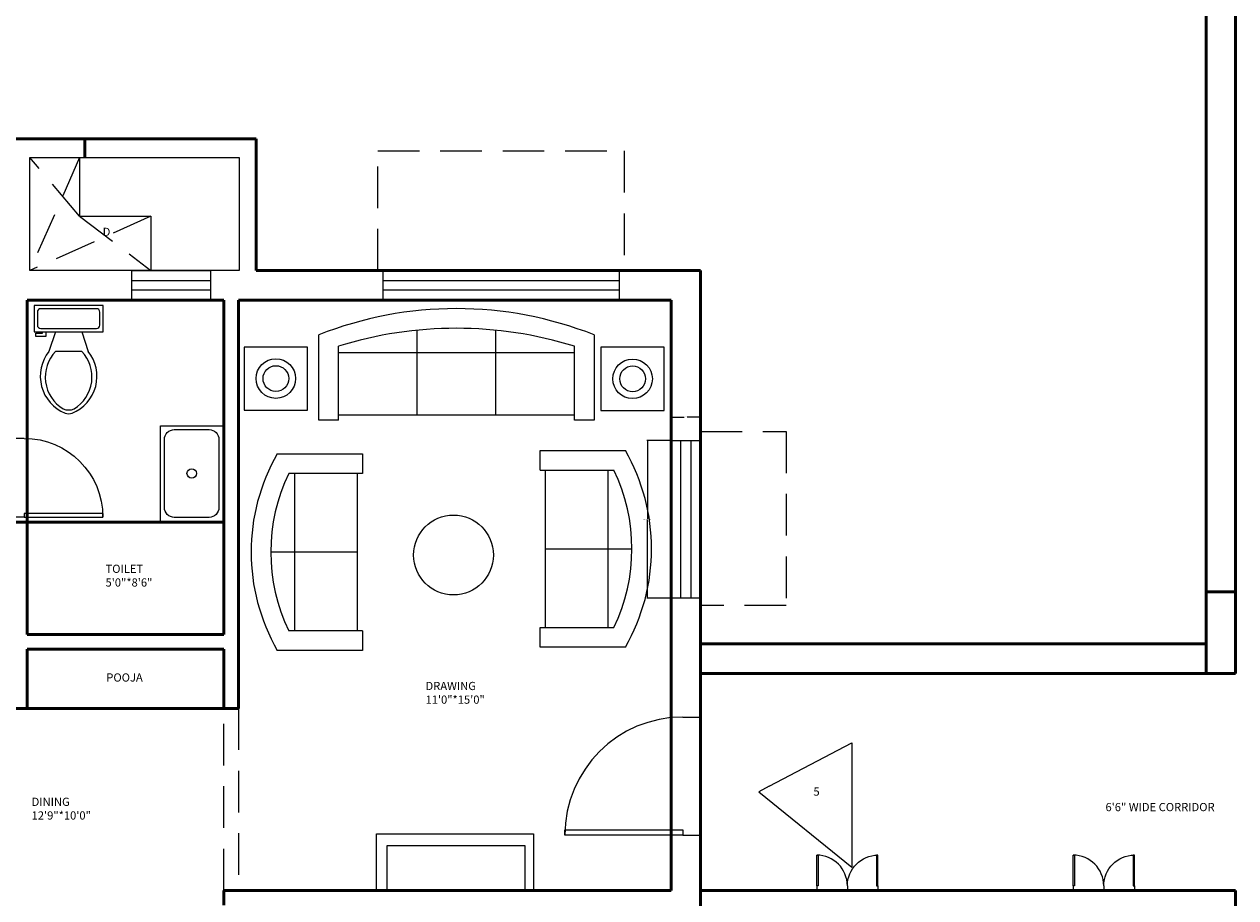
# Model space of a CAD drawing. Units: inches. Extents: x 4795 to 6024, y 2716 to 5025.
# Tile 6 of 19: x 5081 to 5450, y 3549 to 3816. Entities that reach past the tile are written whole.
import ezdxf

# ---------------------------------------------------------------- set-up
doc = ezdxf.new("R2010")
doc.units = ezdxf.units.IN
doc.linetypes.add('DASHED', pattern=[19.05, 12.7, -6.35])
for name, color, linetype, lineweight in [('A-ANNO-DIMS', 2, 'Continuous', 18), ('A-ANNO-TEXT', 7, 'Continuous', 18), ('A-AREA-IDEN', 3, 'Continuous', 18), ('A-DOOR', 4, 'Continuous', 25), ('A-FLOR-FIXT', 9, 'Continuous', 18), ('A-FURN', 8, 'Continuous', 18), ('A-GLAZ', 4, 'Continuous', 25), ('A-WALL', 7, 'Continuous', 50), ('A-WALL-OVHD', 8, 'DASHED', 18)]:
    doc.layers.add(name, color=color, linetype=linetype, lineweight=lineweight)
doc.styles.get("Standard").update_dxf_attribs({"font": 'arial.ttf'})
doc.dimstyles.get("Standard").update_dxf_attribs({"dimtxt": 0.18, "dimasz": 0.18, "dimexe": 0.18, "dimexo": 0.0625, "dimgap": 0.09, "dimtad": 0, "dimtih": 1, "dimtoh": 1, "dimdec": 4, "dimzin": 0, "dimdsep": 46, "dimtxsty": 'Standard', "dimcen": 0.09, "dimadec": 0, "dimazin": 0, "dimtfac": 1, "dimtdec": 4, "dimtofl": 0, "dimtmove": 0, "dimatfit": 3, "dimfxl": 1, "dimtolj": 1, "dimtzin": 0, "dimarcsym": 0})

# ---------------------------------------------------------------- blocks, each defined once
blk = doc.blocks.new('*U2')
for p, q in [((0, 0), (0, -6)), ((40, 0), (40, -6))]:
    blk.add_line(p, q)
blk.add_lwpolyline([(0, 0), (0, 40), (1.75, 40), (1.75, 0)], close=True)
blk.add_arc((0, 0), 40, 0, 90)
blk = doc.blocks.new('Sofa - Roundback 7 ft.')
for p, q in [((-12.00002, -32.4421), (-12.00003, -6.5971)), ((11.99997, -32.4421), (11.99998, -6.5971)), ((-36.000027, -34), (-36.000027, -11.4696)), ((-35.999844, -13.3819), (35.9998, -13.3819)), ((35.99998, -34), (35.99998, -11.4696)), ((-36.000027, -32.4421), (35.99998, -32.4421))]:
    blk.add_line(p, q)
for points in [[(-36.000027, -34), (-42.000027, -34), (-42.000027, -8)], [(41.99998, -8), (41.99998, -34), (35.99998, -34)]]:
    blk.add_lwpolyline(points)
for centre, radius, start, end in [((0, -114.25), 114.25, 68.43141, 111.5686), ((-0.00001, -127.1968), 121.1968, 72.72033, 107.2797)]:
    blk.add_arc(centre, radius, start, end)
blk = doc.blocks.new('Sofa - Roundback Loveseat 5 ft.')
for p, q in [((0, -32.44198), (0, -5.99998)), ((-24, -33.99998), (-24, -11.46958)), ((-23.9998, -13.38178), (23.99986, -13.38178)), ((24.00004, -33.99998), (24.00004, -11.46958)), ((-24, -32.44198), (24.00004, -32.44198))]:
    blk.add_line(p, q)
for points in [[(-24, -33.99998), (-30, -33.99998), (-30, -7.99998)], [(30.00004, -7.99998), (30.00004, -33.99998), (24.00004, -33.99998)]]:
    blk.add_lwpolyline(points)
for centre, radius, start, end in [((0, -60.24998), 60.24998, 60.13715, 119.8628), ((0, -61.38438), 55.38444, 64.32083, 115.6792)]:
    blk.add_arc(centre, radius, start, end)
blk = doc.blocks.new('Toilet - top')
for p, q in [((9.5, -6), (9.5, -2)), ((-10, -8.5), (-8, -8.5)), ((-10, -9.5), (-10, -8.5)), ((-7, -9.5), (-10, -9.5)), ((-8, -8.5), (-8, -8)), ((-7, -8), (-7, -9.5)), ((-4, -8), (-6, -14)), ((4, -8), (6, -14)), ((4, -14), (-4, -14))]:
    blk.add_line(p, q)
blk.add_lwpolyline([(10.5, -8), (10.5, 0), (-10.5, 0), (-10.5, -8)], close=True)
for points in [[(-9.5, -2), (-9.5, -6)], [(8.5, -1), (-8.5, -1)], [(-8.5, -7), (8.5, -7)]]:
    blk.add_lwpolyline(points)
for centre, radius, start, end in [((-8.62, -1.88), 0.884, 81.8699, 188.1301), ((8.62, -1.88), 0.884, 351.8699, 98.1301), ((-8.62, -6.12), 0.884, 171.8699, 278.1301), ((8.62, -6.12), 0.884, 261.8699, 8.1301), ((3.52, -21.58), 12.17, 141.4691, 247.9714), ((4.2, -21.82), 11.33, 136.3677, 238.9468), ((-3.52, -21.58), 12.17, 292.0284, 38.5307), ((-4.2, -21.82), 11.33, 301.053, 43.6321), ((0, -27.88), 4, 245.7318, 294.2682), ((0, -29), 4, 254.8605, 285.1395)]:
    blk.add_arc(centre, radius, start, end)
blk = doc.blocks.new('WIN-48')
for p, q in [((0, 0), (0, 48)), ((0, 48), (9, 48)), ((3, 0), (3, 48)), ((6, 48), (6, 0)), ((9, 48), (9, 0)), ((9, 0), (0, 0))]:
    blk.add_line(p, q)
blk = doc.blocks.new('WIN-72')
for p, q in [((0, 0), (0, 9)), ((0, 9), (72, 9)), ((72, 9), (72, 0)), ((0, 6), (72, 6)), ((72, 3), (0, 3)), ((72, 0), (0, 0))]:
    blk.add_line(p, q)
blk = doc.blocks.new('WIN-24')
for p, q in [((0, 0), (0, 9)), ((0, 9), (24, 9)), ((24, 9), (24, 0)), ((0, 6), (24, 6)), ((24, 3), (0, 3)), ((24, 0), (0, 0))]:
    blk.add_line(p, q)
blk = doc.blocks.new('*D35')
at = {"layer": 'A-ANNO-DIMS', "color": 0, "lineweight": -2, "transparency": 16777216}
for p, q in [((5277.91, 3688.56), (5270.59, 3688.56)), ((5270.77, 3688.38), (5270.77, 3664.74)), ((5270.77, 3640.74), (5270.77, 3664.38)), ((5277.91, 3640.56), (5270.59, 3640.56))]:
    blk.add_line(p, q, dxfattribs=at)
at = {"layer": 'A-ANNO-DIMS', "color": 0, "lineweight": 100, "transparency": 16777216}
for points in [[(5270.74, 3688.38), (5270.8, 3688.38), (5270.77, 3688.56)], [(5270.74, 3640.74), (5270.8, 3640.74), (5270.77, 3640.56)]]:
    blk.add_solid(points, dxfattribs=at)
at = {"layer": 'DEFPOINTS', "color": 0, "lineweight": 100, "transparency": 16777216}
for p in [(5277.97, 3688.56), (5270.77, 3640.56), (5277.97, 3640.56)]:
    blk.add_point(p, dxfattribs=at)
at = {"layer": 'A-ANNO-DIMS', "color": 0, "transparency": 16777216, "insert": (5270.77, 3664.56), "char_height": 0.18, "attachment_point": 5}
blk.add_mtext('\\A1;WINDOW 4\'-0" 48 TYP.', dxfattribs=at)
blk = doc.blocks.new('*D36')
at = {"layer": 'A-ANNO-DIMS', "color": 0, "lineweight": -2, "transparency": 16777216}
for p, q in [((5277.97, 3688.62), (5277.97, 3695.94)), ((5278.15, 3695.76), (5282.01, 3695.76)), ((5286.79, 3695.76), (5282.93, 3695.76)), ((5286.97, 3688.62), (5286.97, 3695.94))]:
    blk.add_line(p, q, dxfattribs=at)
at = {"layer": 'A-ANNO-DIMS', "color": 0, "lineweight": 100, "transparency": 16777216}
for points in [[(5278.15, 3695.79), (5278.15, 3695.73), (5277.97, 3695.76)], [(5286.79, 3695.79), (5286.79, 3695.73), (5286.97, 3695.76)]]:
    blk.add_solid(points, dxfattribs=at)
at = {"layer": 'DEFPOINTS', "color": 0, "lineweight": 100, "transparency": 16777216}
for p in [(5277.97, 3695.76), (5277.97, 3688.56), (5286.97, 3688.56)]:
    blk.add_point(p, dxfattribs=at)
at = {"layer": 'A-ANNO-DIMS', "color": 0, "transparency": 16777216, "insert": (5282.47, 3695.76), "char_height": 0.18, "attachment_point": 5}
blk.add_mtext('\\A1;9 TYP.', dxfattribs=at)

msp = doc.modelspace()

# ---------------------------------------------------------------- linework, layer by layer
at = {"layer": 'A-FLOR-FIXT'}
msp.add_lwpolyline([(5141.47, 3663.74), (5122.16, 3663.74), (5122.16, 3693.07), (5141.47, 3693.07)], close=True, dxfattribs=at)
msp.add_lwpolyline([(5126.37, 3691.93), (5136.99, 3691.93, -0.414214), (5139.99, 3688.93), (5139.99, 3668.17, -0.414214), (5136.99, 3665.17), (5126.37, 3665.17, -0.414214), (5123.37, 3668.17), (5123.37, 3688.93, -0.414214)], format="xyb", close=True, dxfattribs=at)
msp.add_circle((5131.68, 3678.55), 1.44, dxfattribs=at)
at = {"layer": 'A-FURN'}
for p, q in [((5082.32, 3740.43), (5082.32, 3774.86)), ((5082.32, 3774.86), (5146.16, 3774.86)), ((5097.44, 3774.86), (5097.44, 3757.06)), ((5146.16, 3774.86), (5146.16, 3740.43)), ((5097.44, 3757.06), (5119.25, 3757.06)), ((5119.25, 3757.06), (5119.25, 3740.43)), ((5146.16, 3740.43), (5082.32, 3740.43)), ((5307.95, 3583.17), (5333.15, 3596.44)), ((5333.15, 3596.44), (5333.15, 3558.52)), ((5307.95, 3583.17), (5304.79, 3581.51)), ((5304.79, 3581.51), (5333.15, 3558.52)), ((5188.04, 3551.43), (5188.04, 3568.62)), ((5188.04, 3568.62), (5236.04, 3568.62)), ((5236.04, 3568.62), (5236.04, 3551.43)), ((5191.33, 3551.43), (5191.33, 3565.1)), ((5191.33, 3565.1), (5233.37, 3565.1)), ((5233.37, 3565.1), (5233.37, 3551.43))]:
    msp.add_line(p, q, dxfattribs=at)
for points in [[(5167.05, 3717.11), (5147.69, 3717.11), (5147.69, 3697.86), (5167.05, 3697.86)], [(5275.91, 3717.03), (5256.55, 3717.03), (5256.55, 3697.78), (5275.91, 3697.78)]]:
    msp.add_lwpolyline(points, close=True, dxfattribs=at)
for centre, radius in [((5157.37, 3707.49), 6.04), ((5266.23, 3707.41), 6.04), ((5157.37, 3707.49), 3.92), ((5266.23, 3707.41), 3.92), ((5211.58, 3653.69), 12.16)]:
    msp.add_circle(centre, radius, dxfattribs=at)
at = {"layer": 'A-WALL'}
for p, q in [((5450.22, 4167.14), (5450.22, 3676.49)), ((5441.22, 4158.14), (5441.22, 3676.49)), ((5076.97, 3780.56), (5151.39, 3780.56)), ((5099.08, 3780.56), (5099.08, 3774.86)), ((5151.39, 3780.56), (5151.39, 3740.43)), ((5286.97, 3740.43), (5151.39, 3740.43)), ((5286.97, 3740.43), (5286.97, 3350.43)), ((5081.47, 3731.43), (5081.47, 3629.43)), ((5141.47, 3731.43), (5081.47, 3731.43)), ((5141.47, 3731.43), (5141.47, 3629.43)), ((5277.97, 3731.43), (5145.97, 3731.43)), ((5145.97, 3731.43), (5145.97, 3606.93)), ((5277.97, 3731.43), (5277.97, 3551.43)), ((5441.22, 3676.49), (5441.22, 3626.6)), ((5450.22, 3676.49), (5450.22, 3617.6)), ((5076.97, 3663.74), (5141.47, 3663.74)), ((5441.22, 3642.5), (5450.3, 3642.5)), ((5141.47, 3629.43), (5081.47, 3629.43)), ((5141.47, 3624.93), (5081.47, 3624.93)), ((5081.47, 3624.93), (5081.47, 3606.93)), ((5141.47, 3624.93), (5141.47, 3606.93)), ((5441.22, 3626.6), (5286.97, 3626.6)), ((5441.22, 3626.6), (5441.22, 3617.6)), ((5450.22, 3617.6), (5286.97, 3617.6)), ((5081.47, 3606.93), (5074.88, 3606.93)), ((5081.47, 3606.93), (5145.97, 3606.93)), ((5277.97, 3551.43), (5141.47, 3551.43)), ((5141.47, 3551.43), (5141.47, 3546.93)), ((5286.97, 3551.43), (5450.22, 3551.43)), ((5450.22, 3551.43), (5450.22, 3464.24))]:
    msp.add_line(p, q, dxfattribs=at)
at = {"layer": 'A-WALL-OVHD'}
for p, q in [((5097.44, 3757.06), (5082.32, 3774.86)), ((5097.44, 3774.86), (5082.32, 3740.43)), ((5188.49, 3740.43), (5188.49, 3776.92)), ((5188.49, 3776.92), (5263.68, 3776.92)), ((5263.68, 3776.92), (5263.68, 3740.43)), ((5119.25, 3757.06), (5082.32, 3740.43)), ((5097.44, 3757.06), (5119.25, 3740.43)), ((5286.97, 3691.35), (5313.11, 3691.35)), ((5313.11, 3691.35), (5313.11, 3638.32)), ((5313.11, 3638.32), (5286.97, 3638.32)), ((5141.47, 3551.43), (5141.47, 3606.93)), ((5145.97, 3606.93), (5145.97, 3551.43))]:
    msp.add_line(p, q, dxfattribs=at)

# ---------------------------------------------------------------- block references
at = {"layer": 'A-DOOR'}
for p, xscale, yscale, zscale, rotation in [((5080.57, 3665.26), -0.6, 0.6, 0.6, 270), ((5281.57, 3568.28), 0.9, 0.9, 0.9, 90)]:
    msp.add_blockref('*U2', p, dxfattribs=dict(at, xscale=xscale, yscale=yscale, zscale=zscale, rotation=rotation))
at = {"layer": 'A-DOOR', "yscale": 0.2337145210718518, "zscale": 0.2337145210718518}
for p, xscale in [((5322.42, 3552.81), 0.2337145210718518), ((5341.12, 3552.81), -0.2337145210718518), ((5400.66, 3552.81), 0.2337145210718518), ((5419.35, 3552.81), -0.2337145210718518)]:
    msp.add_blockref('*U2', p, dxfattribs=dict(at, xscale=xscale))
at = {"layer": 'A-FLOR-FIXT'}
msp.add_blockref('Toilet - top', (5094.13, 3729.79), dxfattribs=at)
at = {"layer": 'A-FURN'}
msp.add_blockref('Sofa - Roundback 7 ft.', (5212.46, 3728.83), dxfattribs=at)
for p, rotation in [((5149.81, 3654.59), 90), ((5272.02, 3655.57), 270)]:
    msp.add_blockref('Sofa - Roundback Loveseat 5 ft.', p, dxfattribs=dict(at, rotation=rotation))
at = {"layer": 'A-GLAZ', "rotation": 180}
for name, p in [('WIN-24', (5137.43, 3740.43)), ('WIN-72', (5262.11, 3740.43)), ('WIN-48', (5286.97, 3688.56))]:
    msp.add_blockref(name, p, dxfattribs=at)

# ---------------------------------------------------------------- texts
at = {"layer": 'A-ANNO-TEXT', "char_height": 2.5, "attachment_point": 1}
for s, width, insert in [('D', 2.4843, (5104.52, 3753.49)), ('5', 9.3052, (5321.42, 3582.79))]:
    msp.add_mtext_dynamic_manual_height_columns(s, width=width, gutter_width=12.5, heights=[0], dxfattribs=dict(at, insert=insert))
at = {"layer": 'A-AREA-IDEN', "char_height": 2.5, "attachment_point": 1}
for s, width, insert in [('TOILET\\P5\'0"*8\'6"', 40.9232, (5105.39, 3650.73)), ('POOJA', 31.2165, (5105.63, 3617.59)), ('DRAWING\\P11\'0"*15\'0"', 55.9517, (5203.04, 3615)), ('DINING\\P12\'9"*10\'0"', 50.5196, (5082.84, 3579.68)), ('6\'6" WIDE CORRIDOR', 138.0689, (5410.54, 3578.07))]:
    msp.add_mtext_dynamic_manual_height_columns(s, width=width, gutter_width=12.5, heights=[0], dxfattribs=dict(at, insert=insert))

# ---------------------------------------------------------------- dimensions: what is measured, and where the dimension line sits
at = {"layer": 'A-ANNO-DIMS'}
for base, p1, p2, angle, text, picture, middle in [((5277.97, 3695.76), (5286.97, 3688.56), (5277.97, 3688.56), 180, '<> TYP.', '*D36', (5282.47, 3695.76)), ((5270.77, 3640.56), (5277.97, 3688.56), (5277.97, 3640.56), 270, 'WINDOW 4\'-0" <> TYP.', '*D35', (5270.77, 3664.56))]:
    dim = msp.add_linear_dim(base=base, p1=p1, p2=p2, angle=angle, text=text, dimstyle='Standard', override={"dimdec": 0, "dimlfac": 1, "dimrnd": 0, "dimzin": 0, "dimdsep": 46, "dimlunit": 2}, dxfattribs=at)
    dim.commit()
    dim.dimension.update_dxf_attribs({"geometry": picture, "text_midpoint": middle})

doc.saveas('drawing.dxf')
